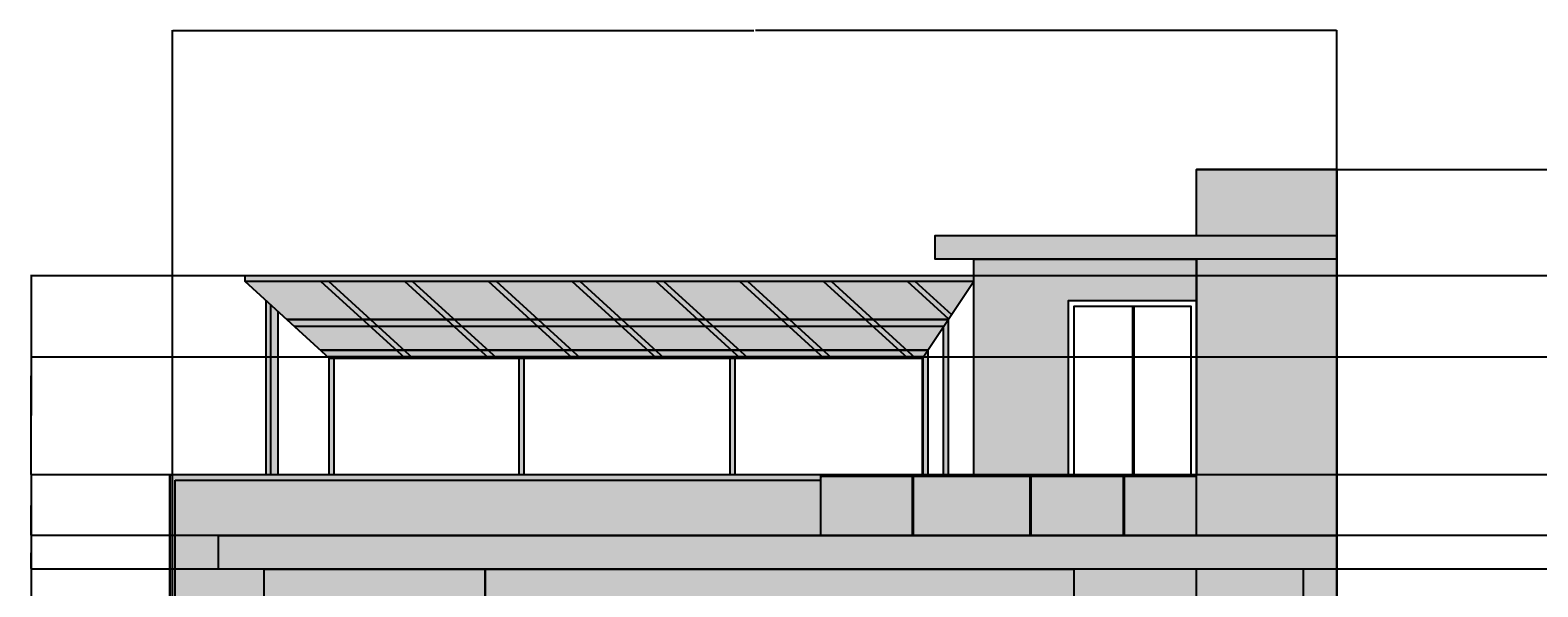
# Model space of a CAD drawing. Units: feet. Extents: x 2193 to 3502, y 890 to 1601.
# Tile 8 of 17: x 2193 to 2848, y 1360 to 1601. Entities that reach past the tile are written whole.
import ezdxf

# ---------------------------------------------------------------- set-up
doc = ezdxf.new("R2010")
doc.units = ezdxf.units.FT
for name, color, linetype, lineweight in [('A-ANNO-DIMS', 2, 'Continuous', 18), ('A-ELEV', 7, 'Continuous', 25), ('A-ELEV-PATT', 8, 'Continuous', 13)]:
    doc.layers.add(name, color=color, linetype=linetype, lineweight=lineweight)
doc.styles.get("Standard").update_dxf_attribs({"font": 'arial.ttf'})
doc.dimstyles.get("Standard").update_dxf_attribs({"dimtxt": 0.18, "dimasz": 0.18, "dimexe": 0.18, "dimexo": 0.0625, "dimgap": 0.09, "dimtad": 0, "dimtih": 1, "dimtoh": 1, "dimdec": 0, "dimzin": 0, "dimdsep": 46, "dimlunit": 3, "dimtxsty": 'Standard', "dimcen": 0.09, "dimadec": 0, "dimazin": 0, "dimtfac": 1, "dimtdec": 0, "dimtofl": 0, "dimtmove": 0, "dimatfit": 3, "dimfxl": 1, "dimtolj": 1, "dimtzin": 0, "dimarcsym": 0})

# ---------------------------------------------------------------- blocks, each defined once
blk = doc.blocks.new('*D20')
at = {"layer": 'A-ANNO-DIMS', "color": 0, "lineweight": -2, "transparency": 16777216}
for p, q in [((2933.15, 1408.48), (2193.56, 1408.48)), ((2193.74, 1408.3), (2193.74, 1240.94)), ((2193.74, 1073.21), (2193.74, 1240.57)), ((2934.31, 1073.03), (2193.56, 1073.03))]:
    blk.add_line(p, q, dxfattribs=at)
at = {"layer": 'A-ANNO-DIMS', "color": 0, "transparency": 16777216}
for points in [[(2193.71, 1408.3), (2193.77, 1408.3), (2193.74, 1408.48)], [(2193.71, 1073.21), (2193.77, 1073.21), (2193.74, 1073.03)]]:
    blk.add_solid(points, dxfattribs=at)
at = {"layer": 'Defpoints', "color": 0, "transparency": 16777216}
for p in [(2193.74, 1408.48), (2933.21, 1408.48), (2934.37, 1073.03)]:
    blk.add_point(p, dxfattribs=at)
at = {"layer": 'A-ANNO-DIMS', "color": 0, "transparency": 16777216, "insert": (2193.74, 1240.76), "char_height": 0.18, "attachment_point": 5}
blk.add_mtext('\\A1;335.45', dxfattribs=at)
blk = doc.blocks.new('*D21')
at = {"layer": 'A-ANNO-DIMS', "color": 0, "lineweight": -2, "transparency": 16777216}
for p, q in [((2965.66, 1494.8), (2193.56, 1494.8)), ((2193.74, 1494.62), (2193.74, 1451.82)), ((2193.74, 1408.66), (2193.74, 1451.46)), ((2974.89, 1408.48), (2193.56, 1408.48))]:
    blk.add_line(p, q, dxfattribs=at)
at = {"layer": 'A-ANNO-DIMS', "color": 0, "transparency": 16777216}
for points in [[(2193.71, 1494.62), (2193.77, 1494.62), (2193.74, 1494.8)], [(2193.71, 1408.66), (2193.77, 1408.66), (2193.74, 1408.48)]]:
    blk.add_solid(points, dxfattribs=at)
at = {"layer": 'Defpoints', "color": 0, "transparency": 16777216}
for p in [(2193.74, 1494.8), (2965.72, 1494.8), (2974.95, 1408.48)]:
    blk.add_point(p, dxfattribs=at)
at = {"layer": 'A-ANNO-DIMS', "color": 0, "transparency": 16777216, "insert": (2193.74, 1451.64), "char_height": 0.18, "attachment_point": 5}
blk.add_mtext('\\A1;86.32', dxfattribs=at)
blk = doc.blocks.new('*D26')
at = {"layer": 'A-ANNO-DIMS', "color": 0, "lineweight": -2, "transparency": 16777216}
for p, q in [((2255.16, 950.89), (2255.16, 1601.47)), ((2255.34, 1601.29), (2507.42, 1601.29)), ((2760.29, 1601.29), (2508.21, 1601.29)), ((2760.47, 1541.11), (2760.47, 1601.47))]:
    blk.add_line(p, q, dxfattribs=at)
at = {"layer": 'A-ANNO-DIMS', "color": 0, "transparency": 16777216}
for points in [[(2255.34, 1601.32), (2255.34, 1601.26), (2255.16, 1601.29)], [(2760.29, 1601.32), (2760.29, 1601.26), (2760.47, 1601.29)]]:
    blk.add_solid(points, dxfattribs=at)
at = {"layer": 'Defpoints', "color": 0, "transparency": 16777216}
for p in [(2760.47, 1601.29), (2760.47, 1541.04), (2255.16, 950.82)]:
    blk.add_point(p, dxfattribs=at)
at = {"layer": 'A-ANNO-DIMS', "color": 0, "transparency": 16777216, "insert": (2507.82, 1601.29), "char_height": 0.18, "attachment_point": 5}
blk.add_mtext('\\A1;505.3', dxfattribs=at)
blk = doc.blocks.new('*D31')
at = {"layer": 'A-ANNO-DIMS', "color": 0, "lineweight": -2, "transparency": 16777216}
for p, q in [((2760.54, 1541.04), (3501.85, 1541.04)), ((3501.67, 1540.86), (3501.67, 1246.12)), ((3501.67, 951), (3501.67, 1245.75)), ((2762.27, 950.82), (3501.85, 950.82))]:
    blk.add_line(p, q, dxfattribs=at)
at = {"layer": 'A-ANNO-DIMS', "color": 0, "transparency": 16777216}
for points in [[(3501.64, 1540.86), (3501.7, 1540.86), (3501.67, 1541.04)], [(3501.64, 951), (3501.7, 951), (3501.67, 950.82)]]:
    blk.add_solid(points, dxfattribs=at)
at = {"layer": 'Defpoints', "color": 0, "transparency": 16777216}
for p in [(2760.47, 1541.04), (3501.67, 1541.04), (2762.2, 950.82)]:
    blk.add_point(p, dxfattribs=at)
at = {"layer": 'A-ANNO-DIMS', "color": 0, "transparency": 16777216, "insert": (3501.67, 1245.93), "char_height": 0.18, "attachment_point": 5}
blk.add_mtext('\\A1;590.2', dxfattribs=at)
blk = doc.blocks.new('*D33')
at = {"layer": 'A-ANNO-DIMS', "color": 0, "lineweight": -2, "transparency": 16777216}
for p, q in [((2253.93, 1408.48), (2193.56, 1408.48)), ((2193.74, 1408.3), (2193.74, 1240.94)), ((2193.74, 1073.21), (2193.74, 1240.57)), ((2255.09, 1073.03), (2193.56, 1073.03))]:
    blk.add_line(p, q, dxfattribs=at)
at = {"layer": 'A-ANNO-DIMS', "color": 0, "transparency": 16777216}
for points in [[(2193.71, 1408.3), (2193.77, 1408.3), (2193.74, 1408.48)], [(2193.71, 1073.21), (2193.77, 1073.21), (2193.74, 1073.03)]]:
    blk.add_solid(points, dxfattribs=at)
at = {"layer": 'Defpoints', "color": 0, "transparency": 16777216}
for p in [(2193.74, 1408.48), (2253.99, 1408.48), (2255.16, 1073.03)]:
    blk.add_point(p, dxfattribs=at)
at = {"layer": 'A-ANNO-DIMS', "color": 0, "transparency": 16777216, "insert": (2193.74, 1240.76), "char_height": 0.18, "attachment_point": 5}
blk.add_mtext('\\A1;335.45', dxfattribs=at)
blk = doc.blocks.new('*D34')
at = {"layer": 'A-ANNO-DIMS', "color": 0, "lineweight": -2, "transparency": 16777216}
for p, q in [((2286.44, 1494.8), (2193.56, 1494.8)), ((2193.74, 1494.62), (2193.74, 1451.82)), ((2193.74, 1408.66), (2193.74, 1451.46)), ((2295.67, 1408.48), (2193.56, 1408.48))]:
    blk.add_line(p, q, dxfattribs=at)
at = {"layer": 'A-ANNO-DIMS', "color": 0, "transparency": 16777216}
for points in [[(2193.71, 1494.62), (2193.77, 1494.62), (2193.74, 1494.8)], [(2193.71, 1408.66), (2193.77, 1408.66), (2193.74, 1408.48)]]:
    blk.add_solid(points, dxfattribs=at)
at = {"layer": 'Defpoints', "color": 0, "transparency": 16777216}
for p in [(2193.74, 1494.8), (2286.5, 1494.8), (2295.74, 1408.48)]:
    blk.add_point(p, dxfattribs=at)
at = {"layer": 'A-ANNO-DIMS', "color": 0, "transparency": 16777216, "insert": (2193.74, 1451.64), "char_height": 0.18, "attachment_point": 5}
blk.add_mtext('\\A1;86.32', dxfattribs=at)
blk = doc.blocks.new('*D37')
at = {"layer": 'A-ANNO-DIMS', "color": 0, "lineweight": -2, "transparency": 16777216}
for p, q in [((2974.05, 1367.57), (2193.56, 1367.57)), ((2193.74, 1367.39), (2193.74, 1318.3)), ((2193.74, 1268.84), (2193.74, 1317.93)), ((2974.05, 1268.66), (2193.56, 1268.66))]:
    blk.add_line(p, q, dxfattribs=at)
at = {"layer": 'A-ANNO-DIMS', "color": 0, "transparency": 16777216}
for points in [[(2193.71, 1367.39), (2193.77, 1367.39), (2193.74, 1367.57)], [(2193.71, 1268.84), (2193.77, 1268.84), (2193.74, 1268.66)]]:
    blk.add_solid(points, dxfattribs=at)
at = {"layer": 'Defpoints', "color": 0, "transparency": 16777216}
for p in [(2193.74, 1367.57), (2974.12, 1367.57), (2974.12, 1268.66)]:
    blk.add_point(p, dxfattribs=at)
at = {"layer": 'A-ANNO-DIMS', "color": 0, "transparency": 16777216, "insert": (2193.74, 1318.12), "char_height": 0.18, "attachment_point": 5}
blk.add_mtext('\\A1;98.91', dxfattribs=at)
blk = doc.blocks.new('*D38')
at = {"layer": 'A-ANNO-DIMS', "color": 0, "lineweight": -2, "transparency": 16777216}
for p, q in [((2954.2, 1382.08), (2193.56, 1382.08)), ((2193.74, 1381.9), (2193.74, 1375.01)), ((2193.74, 1367.75), (2193.74, 1374.64)), ((2954.2, 1367.57), (2193.56, 1367.57))]:
    blk.add_line(p, q, dxfattribs=at)
at = {"layer": 'A-ANNO-DIMS', "color": 0, "transparency": 16777216}
for points in [[(2193.71, 1381.9), (2193.77, 1381.9), (2193.74, 1382.08)], [(2193.71, 1367.75), (2193.77, 1367.75), (2193.74, 1367.57)]]:
    blk.add_solid(points, dxfattribs=at)
at = {"layer": 'Defpoints', "color": 0, "transparency": 16777216}
for p in [(2193.74, 1382.08), (2954.26, 1382.08), (2954.26, 1367.57)]:
    blk.add_point(p, dxfattribs=at)
at = {"layer": 'A-ANNO-DIMS', "color": 0, "transparency": 16777216, "insert": (2193.74, 1374.83), "char_height": 0.18, "attachment_point": 5}
blk.add_mtext('\\A1;14.502', dxfattribs=at)
blk = doc.blocks.new('*D39')
at = {"layer": 'A-ANNO-DIMS', "color": 0, "lineweight": -2, "transparency": 16777216}
for p, q in [((2933.15, 1408.48), (2193.56, 1408.48)), ((2193.74, 1408.3), (2193.74, 1395.46)), ((2193.74, 1382.26), (2193.74, 1395.1)), ((2954.2, 1382.08), (2193.56, 1382.08))]:
    blk.add_line(p, q, dxfattribs=at)
at = {"layer": 'A-ANNO-DIMS', "color": 0, "transparency": 16777216}
for points in [[(2193.71, 1408.3), (2193.77, 1408.3), (2193.74, 1408.48)], [(2193.71, 1382.26), (2193.77, 1382.26), (2193.74, 1382.08)]]:
    blk.add_solid(points, dxfattribs=at)
at = {"layer": 'Defpoints', "color": 0, "transparency": 16777216}
for p in [(2193.74, 1408.48), (2933.21, 1408.48), (2954.26, 1382.08)]:
    blk.add_point(p, dxfattribs=at)
at = {"layer": 'A-ANNO-DIMS', "color": 0, "transparency": 16777216, "insert": (2193.74, 1395.28), "char_height": 0.18, "attachment_point": 5}
blk.add_mtext('\\A1;26.405', dxfattribs=at)
blk = doc.blocks.new('*D58')
at = {"layer": 'A-ANNO-DIMS', "color": 0, "lineweight": -2, "transparency": 16777216}
for p, q in [((3001.83, 1459.6), (2193.56, 1459.6)), ((2193.74, 1459.42), (2193.74, 1434.22)), ((2193.74, 1408.66), (2193.74, 1433.86)), ((2974.89, 1408.48), (2193.56, 1408.48))]:
    blk.add_line(p, q, dxfattribs=at)
at = {"layer": 'A-ANNO-DIMS', "color": 0, "transparency": 16777216}
for points in [[(2193.71, 1459.42), (2193.77, 1459.42), (2193.74, 1459.6)], [(2193.71, 1408.66), (2193.77, 1408.66), (2193.74, 1408.48)]]:
    blk.add_solid(points, dxfattribs=at)
at = {"layer": 'Defpoints', "color": 0, "transparency": 16777216}
for p in [(2193.74, 1459.6), (3001.89, 1459.6), (2974.95, 1408.48)]:
    blk.add_point(p, dxfattribs=at)
at = {"layer": 'A-ANNO-DIMS', "color": 0, "transparency": 16777216, "insert": (2193.74, 1434.04), "char_height": 0.18, "attachment_point": 5}
blk.add_mtext('\\A1;51.12', dxfattribs=at)

msp = doc.modelspace()

# ---------------------------------------------------------------- hatches: boundary and pattern name
at = {"layer": 'A-ELEV-PATT'}
h = msp.add_hatch(color=256, dxfattribs=at)
h.dxf.hatch_style = 1
h.paths.add_polyline_path([(2760.4733, 1541.0441), (2699.6322, 1541.0441), (2699.6322, 1512.3957), (2760.4733, 1512.3957)])
h.paths.add_polyline_path([(2760.4733, 1502.0763), (2699.6322, 1502.0763), (2699.6322, 1382.0763), (2760.4733, 1382.0763)])
h.paths.add_polyline_path([(2745.971, 1367.5739), (2699.6322, 1367.5739), (2699.6322, 1089.3627), (2760.4733, 1089.3627), (2760.4733, 1166.2327), (2745.971, 1166.2327)])
h.paths.add_polyline_path([(2754.7661, 1011.1246), (2690.9216, 1011.1246), (2690.9216, 993.3923), (2754.7661, 993.3923)])
h.paths.add_polyline_path([(2689.6008, 1011.1246), (2625.7563, 1011.1246), (2625.7563, 993.3923), (2689.6008, 993.3923)])
h.paths.add_polyline_path([(2599.6883, 1249.8256), (2598.591, 1249.8256), (2598.591, 1233.561), (2599.6883, 1233.561)])
h.paths.add_polyline_path([(2602.5204, 1247.0422), (2601.423, 1247.0422), (2601.423, 1233.561), (2602.5204, 1233.561)])
h.paths.add_polyline_path([(2606.5316, 1250.4403), (2605.4342, 1250.4403), (2605.4342, 1233.561), (2606.5316, 1233.561)])
h.paths.add_polyline_path([(2609.5836, 1248.4363), (2608.4862, 1248.4363), (2608.4862, 1233.561), (2609.5836, 1233.561)])
h.paths.add_polyline_path([(2613.8564, 1243.2956), (2612.759, 1243.2956), (2612.759, 1233.561), (2613.8564, 1233.561)])
h.paths.add_polyline_path([(2616.5596, 1249.6561), (2615.4622, 1249.6561), (2615.4622, 1233.561), (2616.5596, 1233.561)])
h.paths.add_polyline_path([(2599.6883, 1233.561), (2598.591, 1233.561), (2598.591, 1224.865), (2599.6883, 1224.865)])
h.paths.add_polyline_path([(2602.5204, 1233.561), (2601.423, 1233.561), (2601.423, 1224.865), (2602.5204, 1224.865)])
h.paths.add_polyline_path([(2606.5316, 1233.561), (2605.4342, 1233.561), (2605.4342, 1224.865), (2606.5316, 1224.865)])
h.paths.add_polyline_path([(2609.5836, 1233.561), (2608.4862, 1233.561), (2608.4862, 1224.865), (2609.5836, 1224.865)])
h.paths.add_polyline_path([(2613.8564, 1233.561), (2612.759, 1233.561), (2612.759, 1224.865), (2613.8564, 1224.865)])
h.paths.add_polyline_path([(2616.5596, 1233.561), (2615.4622, 1233.561), (2615.4622, 1224.865), (2616.5596, 1224.865)])
h.paths.add_polyline_path([(2599.6883, 1224.865), (2598.591, 1224.865), (2598.591, 1115.2331), (2599.6883, 1115.2331)])
h.paths.add_polyline_path([(2602.5204, 1224.865), (2601.423, 1224.865), (2601.423, 1112.4498), (2602.5204, 1112.4498)])
h.paths.add_polyline_path([(2606.5316, 1224.865), (2605.4342, 1224.865), (2605.4342, 1115.8479), (2606.5316, 1115.8479)])
h.paths.add_polyline_path([(2609.5836, 1224.865), (2608.4862, 1224.865), (2608.4862, 1113.8439), (2609.5836, 1113.8439)])
h.paths.add_polyline_path([(2616.5596, 1224.865), (2615.4622, 1224.865), (2615.4622, 1115.0637), (2616.5596, 1115.0637)])
h.paths.add_polyline_path([(2613.8564, 1224.865), (2612.759, 1224.865), (2612.759, 1108.7032), (2613.8564, 1108.7032)])
h = msp.add_hatch(color=256, dxfattribs=at)
h.dxf.hatch_style = 1
h.paths.add_polyline_path([(2760.4733, 1512.3957), (2586.1736, 1512.3957), (2586.1736, 1502.0763), (2602.8648, 1502.0763), (2699.5726, 1502.0763), (2699.6322, 1502.0763), (2760.4733, 1502.0763)])
h.paths.add_polyline_path([(2760.4733, 1382.0763), (2275.0482, 1382.0763), (2275.0482, 1367.5739), (2745.971, 1367.5739), (2745.971, 1166.2327), (2760.4733, 1166.2327)])
h.paths.add_polyline_path([(2468.2854, 1266.7092), (2294.8992, 1266.7092), (2294.8992, 1079.031), (2468.2854, 1079.031)])
h.paths.add_polyline_path([(2301.4984, 1260.11), (2461.6863, 1260.11), (2461.6863, 1085.6301), (2301.4984, 1085.6301)], flags=16)
h.paths.add_polyline_path([(2452.7821, 1241.1967), (2452.7821, 1217.2819), (2454.6216, 1217.2819), (2454.6216, 1133.1367), (2461.6863, 1133.1367), (2461.6863, 1132.3937), (2381.7172, 1132.3937), (2381.7172, 1085.6301), (2381.4675, 1085.6301), (2381.4675, 1132.3937), (2301.4984, 1132.3937), (2301.4984, 1133.1367), (2301.4984, 1217.2819), (2390.8933, 1217.2819), (2390.8933, 1241.1967)], flags=0)
h.paths.add_polyline_path([(2372.4936, 1214.8367), (2372.4936, 1133.1367), (2371.1246, 1133.1367), (2371.1246, 1214.8367), (2337.2323, 1214.8367), (2337.2323, 1133.1367), (2335.8632, 1133.1367), (2335.8632, 1214.8367), (2337.2323, 1214.8367)], flags=0)
h = msp.add_hatch(color=256, dxfattribs=at)
h.dxf.hatch_style = 1
h.paths.add_polyline_path([(2390.8933, 1367.5739), (2294.8992, 1367.5739), (2294.8992, 1329.5765), (2390.8933, 1329.5765)])
h.paths.add_polyline_path([(2489.6169, 1055.3069), (2585.8844, 1055.3069), (2585.8844, 1032.1935), (2620.0491, 1032.1935), (2620.0491, 1073.031), (2452.7821, 1073.031), (2452.7821, 1032.1935), (2489.6169, 1032.1935)])
h.paths.add_polyline_path([(2754.7661, 1073.031), (2654.2841, 1073.031), (2654.2841, 1047.0961), (2754.7661, 1047.0961)])
h.paths.add_polyline_path([(2643.9681, 1484.1152), (2699.5726, 1484.1152), (2699.5726, 1502.0763), (2602.8648, 1502.0763), (2602.8648, 1408.4814), (2643.9681, 1408.4814)])
h.paths.add_polyline_path([(2699.6322, 1367.5739), (2646.2844, 1367.5739), (2646.2844, 1268.6599), (2647.1841, 1268.6599), (2647.1841, 1329.5765), (2699.6322, 1329.5765)])
h.paths.add_polyline_path([(2699.6322, 1224.865), (2616.5596, 1224.865), (2616.5596, 1133.8558), (2647.1841, 1133.8558), (2647.1841, 1194.7724), (2699.6322, 1194.7724)])
h = msp.add_hatch(color=256, dxfattribs=at)
h.dxf.hatch_style = 1
h.paths.add_polyline_path([(2760.4733, 956.8829), (2754.7661, 956.8829), (2625.7563, 956.8829), (2626.1971, 953.031), (2626.1971, 950.8228), (2762.2048, 950.8228)])
h.paths.add_polyline_path([(2587.7084, 958.9555), (2461.0056, 958.9555), (2461.0056, 953.031), (2587.7084, 953.031)])
h.paths.add_polyline_path([(2480.0809, 960.0129), (2463.2716, 960.0129), (2461.0056, 958.9555), (2480.0809, 958.9555)])
h.paths.add_polyline_path([(2514.917, 960.0129), (2500.4779, 960.0129), (2500.4779, 958.9555), (2514.917, 958.9555)])
h.paths.add_polyline_path([(2552.6959, 960.0129), (2538.2568, 960.0129), (2538.2568, 958.9555), (2552.6959, 958.9555)])
h.paths.add_polyline_path([(2588.4279, 960.0129), (2573.0929, 960.0129), (2573.0929, 958.9555), (2587.7084, 958.9555)])
h.paths.add_polyline_path([(2588.4279, 960.0129), (2587.7084, 958.9555), (2587.7084, 953.031), (2588.4279, 953.031)])
h.paths.add_polyline_path([(2461.0056, 956.8829), (2261.443, 956.8829), (2255.1574, 953.031), (2461.0056, 953.031)])
h.paths.add_polyline_path([(2625.7563, 956.8829), (2600.3918, 956.8829), (2600.3918, 953.031), (2626.1971, 953.031)])
h.paths.add_polyline_path([(2600.3918, 956.8829), (2588.4279, 956.8829), (2588.4279, 953.031), (2600.3918, 953.031)])
h.paths.add_polyline_path([(2602.8648, 1494.8043), (2286.5029, 1494.8043), (2286.5029, 1492.5146), (2602.8648, 1492.5146)])
h.paths.add_polyline_path([(2322.8578, 1492.5146), (2319.4392, 1492.5146), (2337.7496, 1475.8561), (2341.1681, 1475.8561)])
h.paths.add_polyline_path([(2341.1681, 1475.8561), (2337.7496, 1475.8561), (2341.051, 1472.8525), (2344.4696, 1472.8525)])
h.paths.add_polyline_path([(2344.4696, 1472.8525), (2341.051, 1472.8525), (2352.3124, 1462.6071), (2355.731, 1462.6071)])
h.paths.add_polyline_path([(2355.731, 1462.6071), (2352.3124, 1462.6071), (2355.6139, 1459.6035), (2359.0325, 1459.6035)])
h.paths.add_polyline_path([(2325.1721, 1459.1592), (2323.1659, 1459.1592), (2323.1659, 1408.4814), (2325.1721, 1408.4814)])
h.paths.add_polyline_path([(2297.6937, 1482.3334), (2295.7368, 1484.1138), (2295.7368, 1408.4814), (2297.6937, 1408.4814)])
h.paths.add_polyline_path([(2300.8766, 1479.4377), (2297.6937, 1482.3334), (2297.6937, 1408.4814), (2300.8766, 1408.4814)])
h.paths.add_polyline_path([(2337.7496, 1475.8561), (2304.8133, 1475.8561), (2308.1148, 1472.8525), (2341.051, 1472.8525)])
h.paths.add_polyline_path([(2352.3124, 1462.6071), (2319.3762, 1462.6071), (2322.6776, 1459.6035), (2355.6139, 1459.6035)])
h.paths.add_polyline_path([(2374.1044, 1475.8561), (2341.1681, 1475.8561), (2344.4696, 1472.8525), (2377.4059, 1472.8525)])
h.paths.add_polyline_path([(2388.6672, 1462.6071), (2355.731, 1462.6071), (2359.0325, 1459.6035), (2391.9687, 1459.6035)])
h.paths.add_polyline_path([(2392.0858, 1462.6071), (2388.6672, 1462.6071), (2391.9687, 1459.6035), (2395.3873, 1459.6035)])
h.paths.add_polyline_path([(2380.8245, 1472.8525), (2377.4059, 1472.8525), (2388.6672, 1462.6071), (2392.0858, 1462.6071)])
h.paths.add_polyline_path([(2377.523, 1475.8561), (2374.1044, 1475.8561), (2377.4059, 1472.8525), (2380.8245, 1472.8525)])
h.paths.add_polyline_path([(2359.2126, 1492.5146), (2355.794, 1492.5146), (2374.1044, 1475.8561), (2377.523, 1475.8561)])
h.paths.add_polyline_path([(2395.5674, 1492.5146), (2392.1488, 1492.5146), (2410.4592, 1475.8561), (2413.8778, 1475.8561)])
h.paths.add_polyline_path([(2410.4592, 1475.8561), (2377.523, 1475.8561), (2380.8245, 1472.8525), (2413.7607, 1472.8525)])
h.paths.add_polyline_path([(2413.8778, 1475.8561), (2410.4592, 1475.8561), (2413.7607, 1472.8525), (2417.1793, 1472.8525)])
h.paths.add_polyline_path([(2417.1793, 1472.8525), (2413.7607, 1472.8525), (2425.022, 1462.6071), (2428.4406, 1462.6071)])
h.paths.add_polyline_path([(2425.022, 1462.6071), (2392.0858, 1462.6071), (2395.3873, 1459.6035), (2428.3235, 1459.6035)])
h.paths.add_polyline_path([(2428.4406, 1462.6071), (2425.022, 1462.6071), (2428.3235, 1459.6035), (2431.7421, 1459.6035)])
h.paths.add_polyline_path([(2461.3769, 1462.6071), (2428.4406, 1462.6071), (2431.7421, 1459.6035), (2464.6784, 1459.6035)])
h.paths.add_polyline_path([(2577.3415, 1492.5146), (2573.9229, 1492.5146), (2591.9256, 1476.1361), (2593.2177, 1478.0707)])
h.paths.add_polyline_path([(2540.9867, 1492.5146), (2537.5681, 1492.5146), (2555.8785, 1475.8561), (2559.2971, 1475.8561)])
h.paths.add_polyline_path([(2591.7386, 1475.8561), (2559.2971, 1475.8561), (2562.5986, 1472.8525), (2589.7325, 1472.8525)])
h.paths.add_polyline_path([(2555.8785, 1475.8561), (2522.9423, 1475.8561), (2526.2437, 1472.8525), (2559.18, 1472.8525)])
h.paths.add_polyline_path([(2559.2971, 1475.8561), (2555.8785, 1475.8561), (2559.18, 1472.8525), (2562.5986, 1472.8525)])
h.paths.add_polyline_path([(2562.5986, 1472.8525), (2559.18, 1472.8525), (2570.4413, 1462.6071), (2573.8599, 1462.6071)])
h.paths.add_polyline_path([(2570.4413, 1462.6071), (2537.5051, 1462.6071), (2540.8066, 1459.6035), (2573.7428, 1459.6035)])
h.paths.add_polyline_path([(2582.8896, 1462.6071), (2573.8599, 1462.6071), (2577.1614, 1459.6035), (2580.8835, 1459.6035)])
h.paths.add_polyline_path([(2573.8599, 1462.6071), (2570.4413, 1462.6071), (2573.7428, 1459.6035), (2577.1614, 1459.6035)])
h.paths.add_polyline_path([(2591.7386, 1475.8561), (2589.7325, 1472.8525), (2589.7325, 1408.4814), (2591.7386, 1408.4814)])
h.paths.add_polyline_path([(2582.8896, 1462.6071), (2580.8835, 1459.6035), (2580.8835, 1408.4814), (2582.8896, 1408.4814)])
h.paths.add_polyline_path([(2504.6319, 1492.5146), (2501.2133, 1492.5146), (2519.5237, 1475.8561), (2522.9423, 1475.8561)])
h.paths.add_polyline_path([(2534.0865, 1462.6071), (2501.1503, 1462.6071), (2504.4518, 1459.6035), (2537.388, 1459.6035)])
h.paths.add_polyline_path([(2537.5051, 1462.6071), (2534.0865, 1462.6071), (2537.388, 1459.6035), (2540.8066, 1459.6035)])
h.paths.add_polyline_path([(2526.2437, 1472.8525), (2522.8252, 1472.8525), (2534.0865, 1462.6071), (2537.5051, 1462.6071)])
h.paths.add_polyline_path([(2522.9423, 1475.8561), (2519.5237, 1475.8561), (2522.8252, 1472.8525), (2526.2437, 1472.8525)])
h.paths.add_polyline_path([(2519.5237, 1475.8561), (2486.5874, 1475.8561), (2489.8889, 1472.8525), (2522.8252, 1472.8525)])
h.paths.add_polyline_path([(2483.1689, 1475.8561), (2450.2326, 1475.8561), (2453.5341, 1472.8525), (2486.4703, 1472.8525)])
h.paths.add_polyline_path([(2486.5874, 1475.8561), (2483.1689, 1475.8561), (2486.4703, 1472.8525), (2489.8889, 1472.8525)])
h.paths.add_polyline_path([(2468.277, 1492.5146), (2464.8585, 1492.5146), (2483.1689, 1475.8561), (2486.5874, 1475.8561)])
h.paths.add_polyline_path([(2489.8889, 1472.8525), (2486.4703, 1472.8525), (2497.7317, 1462.6071), (2501.1503, 1462.6071)])
h.paths.add_polyline_path([(2497.7317, 1462.6071), (2464.7955, 1462.6071), (2468.0969, 1459.6035), (2501.0332, 1459.6035)])
h.paths.add_polyline_path([(2501.1503, 1462.6071), (2497.7317, 1462.6071), (2501.0332, 1459.6035), (2504.4518, 1459.6035)])
h.paths.add_polyline_path([(2464.7955, 1462.6071), (2461.3769, 1462.6071), (2464.6784, 1459.6035), (2468.0969, 1459.6035)])
h.paths.add_polyline_path([(2453.5341, 1472.8525), (2450.1155, 1472.8525), (2461.3769, 1462.6071), (2464.7955, 1462.6071)])
h.paths.add_polyline_path([(2431.9222, 1492.5146), (2428.5036, 1492.5146), (2446.814, 1475.8561), (2450.2326, 1475.8561)])
h.paths.add_polyline_path([(2446.814, 1475.8561), (2413.8778, 1475.8561), (2417.1793, 1472.8525), (2450.1155, 1472.8525)])
h.paths.add_polyline_path([(2450.2326, 1475.8561), (2446.814, 1475.8561), (2450.1155, 1472.8525), (2453.5341, 1472.8525)])
h.paths.add_polyline_path([(2407.5925, 1459.1592), (2405.5863, 1459.1592), (2405.5863, 1408.4814), (2407.5925, 1408.4814)])
h.paths.add_polyline_path([(2499.2252, 1459.1592), (2497.2191, 1459.1592), (2497.2191, 1408.4814), (2499.2252, 1408.4814)])
h = msp.add_hatch(color=256, dxfattribs=at)
h.dxf.hatch_style = 1
h.paths.add_polyline_path([(2319.4392, 1492.5146), (2286.5029, 1492.5146), (2304.8133, 1475.8561), (2337.7496, 1475.8561)])
h.paths.add_polyline_path([(2355.794, 1492.5146), (2322.8578, 1492.5146), (2341.1681, 1475.8561), (2374.1044, 1475.8561)])
h.paths.add_polyline_path([(2392.1488, 1492.5146), (2359.2126, 1492.5146), (2377.523, 1475.8561), (2410.4592, 1475.8561)])
h.paths.add_polyline_path([(2377.4059, 1472.8525), (2344.4696, 1472.8525), (2355.731, 1462.6071), (2388.6672, 1462.6071)])
h.paths.add_polyline_path([(2413.7607, 1472.8525), (2380.8245, 1472.8525), (2392.0858, 1462.6071), (2425.022, 1462.6071)])
h.paths.add_polyline_path([(2341.051, 1472.8525), (2308.1148, 1472.8525), (2319.3762, 1462.6071), (2352.3124, 1462.6071)])
h.paths.add_polyline_path([(2428.5036, 1492.5146), (2395.5674, 1492.5146), (2413.8778, 1475.8561), (2446.814, 1475.8561)])
h.paths.add_polyline_path([(2464.8585, 1492.5146), (2431.9222, 1492.5146), (2450.2326, 1475.8561), (2483.1689, 1475.8561)])
h.paths.add_polyline_path([(2450.1155, 1472.8525), (2417.1793, 1472.8525), (2428.4406, 1462.6071), (2461.3769, 1462.6071)])
h.paths.add_polyline_path([(2486.4703, 1472.8525), (2453.5341, 1472.8525), (2464.7955, 1462.6071), (2497.7317, 1462.6071)])
h.paths.add_polyline_path([(2602.8648, 1492.5146), (2577.3415, 1492.5146), (2593.2177, 1478.0707)])
h.paths.add_polyline_path([(2573.9229, 1492.5146), (2540.9867, 1492.5146), (2559.2971, 1475.8561), (2591.7386, 1475.8561), (2591.9256, 1476.1361)])
h.paths.add_polyline_path([(2589.7325, 1472.8525), (2562.5986, 1472.8525), (2573.8599, 1462.6071), (2582.8896, 1462.6071)])
h.paths.add_polyline_path([(2559.18, 1472.8525), (2526.2437, 1472.8525), (2537.5051, 1462.6071), (2570.4413, 1462.6071)])
h.paths.add_polyline_path([(2537.5681, 1492.5146), (2504.6319, 1492.5146), (2522.9423, 1475.8561), (2555.8785, 1475.8561)])
h.paths.add_polyline_path([(2501.2133, 1492.5146), (2468.277, 1492.5146), (2486.5874, 1475.8561), (2519.5237, 1475.8561)])
h.paths.add_polyline_path([(2522.8252, 1472.8525), (2489.8889, 1472.8525), (2501.1503, 1462.6071), (2534.0865, 1462.6071)])
h = msp.add_hatch(color=256, dxfattribs=at)
h.dxf.hatch_style = 1
h.paths.add_polyline_path([(2256.3232, 1406.15), (2536.5416, 1406.15), (2536.5416, 1408.4814), (2253.9917, 1408.4814), (2253.9917, 1089.3627), (2255.1574, 1089.3627), (2256.3232, 1089.3627)])
h = msp.add_hatch(color=256, dxfattribs=at)
h.dxf.hatch_style = 1
h.paths.add_polyline_path([(2576.3428, 1407.7384), (2536.5416, 1407.7384), (2536.5416, 1406.15), (2536.5416, 1382.0763), (2576.3428, 1382.0763)])
h.paths.add_polyline_path([(2627.3548, 1407.7384), (2576.5924, 1407.7384), (2576.5924, 1382.0763), (2627.3548, 1382.0763)])
h.paths.add_polyline_path([(2667.9236, 1407.7384), (2627.6045, 1407.7384), (2627.6045, 1382.0763), (2667.9236, 1382.0763)])
h.paths.add_polyline_path([(2699.6322, 1407.7384), (2668.1733, 1407.7384), (2668.1733, 1382.0763), (2699.6322, 1382.0763)])
h.paths.add_polyline_path([(2497.5717, 1323.2248), (2470.7305, 1323.2248), (2470.7305, 1271.105), (2497.5717, 1271.105)])
h.paths.add_polyline_path([(2577.3219, 1323.2248), (2500.599, 1323.2248), (2500.599, 1271.105), (2577.3219, 1271.105)])
h.paths.add_polyline_path([(2388.4482, 1327.1314), (2343.4244, 1327.1314), (2343.4244, 1268.6599), (2388.4482, 1268.6599)])
h.paths.add_polyline_path([(2342.3682, 1327.1314), (2297.3443, 1327.1314), (2297.3443, 1268.6599), (2342.3682, 1268.6599)])
h.paths.add_polyline_path([(2335.8632, 1214.8367), (2301.4984, 1214.8367), (2301.4984, 1133.1367), (2335.8632, 1133.1367)])
h.paths.add_polyline_path([(2371.1246, 1214.8367), (2337.2323, 1214.8367), (2337.2323, 1133.1367), (2371.1246, 1133.1367)])
h.paths.add_polyline_path([(2390.8933, 1214.8367), (2372.4936, 1214.8367), (2372.4936, 1133.1367), (2390.8933, 1133.1367)])
h.paths.add_polyline_path([(2577.3219, 1188.4208), (2500.599, 1188.4208), (2500.599, 1136.3009), (2577.3219, 1136.3009)])
h.paths.add_polyline_path([(2497.5717, 1188.4208), (2470.7305, 1188.4208), (2470.7305, 1136.3009), (2497.5717, 1136.3009)])
h.paths.add_polyline_path([(2381.4675, 1132.3937), (2301.4984, 1132.3937), (2301.4984, 1085.6301), (2381.4675, 1085.6301)])
h.paths.add_polyline_path([(2461.6863, 1132.3937), (2381.7172, 1132.3937), (2381.7172, 1085.6301), (2461.6863, 1085.6301)])
h.paths.add_polyline_path([(2494.0463, 1133.1128), (2468.2854, 1133.1128), (2468.2854, 1089.3627), (2494.0463, 1089.3627)])
h.paths.add_polyline_path([(2517.7591, 1133.1128), (2494.296, 1133.1128), (2494.296, 1089.3627), (2517.7591, 1089.3627)])
h.paths.add_polyline_path([(2667.9236, 1133.1128), (2636.5184, 1133.1128), (2636.5184, 1089.3627), (2667.9236, 1089.3627)])
h.paths.add_polyline_path([(2699.6322, 1133.1128), (2668.1733, 1133.1128), (2668.1733, 1089.3627), (2699.6322, 1089.3627)])
h.paths.add_polyline_path([(2651.839, 1070.5859), (2638.7977, 1070.5859), (2638.7977, 1047.0961), (2651.839, 1047.0961)])
h.paths.add_polyline_path([(2637.6317, 1070.5859), (2625.7563, 1070.5859), (2625.7563, 1047.0961), (2637.6317, 1047.0961)])
h.paths.add_polyline_path([(2583.4393, 1052.8618), (2515.9216, 1052.8618), (2515.9216, 1032.1935), (2583.4393, 1032.1935)])
h.paths.add_polyline_path([(2514.4293, 1052.8618), (2492.062, 1052.8618), (2492.062, 1032.1935), (2514.4293, 1032.1935)])
h.paths.add_polyline_path([(2388.4482, 1038.8658), (2348.7682, 1038.8658), (2348.7682, 988.9597), (2388.4482, 988.9597)])
h.paths.add_polyline_path([(2346.3231, 1038.8658), (2309.0883, 1038.8658), (2309.0883, 988.9597), (2346.3231, 988.9597)])
h.paths.add_polyline_path([(2667.9236, 1267.9169), (2636.5184, 1267.9169), (2636.5184, 1241.1967), (2667.9236, 1241.1967)])
h.paths.add_polyline_path([(2699.6322, 1267.9169), (2668.1733, 1267.9169), (2668.1733, 1241.1967), (2699.6322, 1241.1967)])
h.paths.add_polyline_path([(2517.7591, 1267.9169), (2494.296, 1267.9169), (2494.296, 1241.1967), (2517.7591, 1241.1967)])
h.paths.add_polyline_path([(2494.0463, 1267.9169), (2468.2854, 1267.9169), (2468.2854, 1266.7092), (2468.2854, 1241.1967), (2494.0463, 1241.1967)])
h = msp.add_hatch(color=256, dxfattribs=at)
h.dxf.hatch_style = 1
h.paths.add_polyline_path([(2294.8992, 1367.5739), (2275.0482, 1367.5739), (2275.0482, 1382.0763), (2536.5416, 1382.0763), (2536.5416, 1406.15), (2256.3232, 1406.15), (2256.3232, 1089.3627), (2255.1574, 1089.3627), (2255.1574, 1073.031), (2294.8992, 1073.031)])
h.paths.add_polyline_path([(2517.7591, 1241.1967), (2468.2854, 1241.1967), (2468.2854, 1224.865), (2598.591, 1224.865), (2598.591, 1233.561), (2517.7591, 1233.561)])
h.paths.add_polyline_path([(2699.6322, 1241.1967), (2636.5184, 1241.1967), (2636.5184, 1233.561), (2616.5596, 1233.561), (2616.5596, 1224.865), (2699.6322, 1224.865)])
h.paths.add_polyline_path([(2615.4622, 1233.561), (2613.8564, 1233.561), (2613.8564, 1224.865), (2615.4622, 1224.865)])
h.paths.add_polyline_path([(2612.759, 1233.561), (2609.5836, 1233.561), (2609.5836, 1224.865), (2612.759, 1224.865)])
h.paths.add_polyline_path([(2608.4862, 1233.561), (2606.5316, 1233.561), (2606.5316, 1224.865), (2608.4862, 1224.865)])
h.paths.add_polyline_path([(2605.4342, 1233.561), (2602.5204, 1233.561), (2602.5204, 1224.865), (2605.4342, 1224.865)])
h.paths.add_polyline_path([(2601.423, 1233.561), (2599.6883, 1233.561), (2599.6883, 1224.865), (2601.423, 1224.865)])
h.paths.add_polyline_path([(2517.7591, 1089.3627), (2468.2854, 1089.3627), (2468.2854, 1079.031), (2294.8992, 1079.031), (2294.8992, 1073.031), (2390.8933, 1073.031), (2452.7821, 1073.031), (2760.4733, 1073.031), (2760.4733, 1089.3627), (2699.6322, 1089.3627), (2636.5184, 1089.3627), (2636.5184, 1081.7269), (2517.7591, 1081.7269)])
h = msp.add_hatch(color=256, dxfattribs=at)
h.dxf.hatch_style = 1
h.paths.add_polyline_path([(2452.7821, 1355.2199), (2622.9814, 1355.2199), (2622.9814, 1268.6599), (2646.2844, 1268.6599), (2646.2844, 1367.5739), (2390.8933, 1367.5739), (2390.8933, 1268.6599), (2452.7821, 1268.6599)])
h.paths.add_polyline_path([(2452.7821, 1016.4), (2431.9134, 1016.4), (2431.9134, 1032.1935), (2452.7821, 1032.1935), (2452.7821, 1073.031), (2390.8933, 1073.031), (2390.8933, 956.8829), (2452.7821, 956.8829)])
h.paths.add_polyline_path([(2452.7821, 1241.1967), (2390.8933, 1241.1967), (2390.8933, 1133.1367), (2452.7821, 1133.1367)])
h.paths.add_polyline_path([(2636.5184, 1267.9169), (2517.7591, 1267.9169), (2517.7591, 1233.561), (2598.591, 1233.561), (2598.591, 1249.8256), (2599.6883, 1249.8256), (2599.6883, 1233.561), (2601.423, 1233.561), (2601.423, 1247.0422), (2602.5204, 1247.0422), (2602.5204, 1233.561), (2605.4342, 1233.561), (2605.4342, 1250.4403), (2606.5316, 1250.4403), (2606.5316, 1233.561), (2608.4862, 1233.561), (2608.4862, 1248.4363), (2609.5836, 1248.4363), (2609.5836, 1233.561), (2612.759, 1233.561), (2612.759, 1243.2956), (2613.8564, 1243.2956), (2613.8564, 1233.561), (2615.4622, 1233.561), (2615.4622, 1249.6561), (2616.5596, 1249.6561), (2616.5596, 1233.561), (2636.5184, 1233.561)])
h.paths.add_polyline_path([(2601.423, 1133.1128), (2599.6883, 1133.1128), (2599.6883, 1115.2331), (2598.591, 1115.2331), (2598.591, 1133.1128), (2517.7591, 1133.1128), (2517.7591, 1081.7269), (2636.5184, 1081.7269), (2636.5184, 1133.1128), (2616.5596, 1133.1128), (2616.5596, 1115.0637), (2615.4622, 1115.0637), (2615.4622, 1133.1128), (2613.8564, 1133.1128), (2613.8564, 1108.7032), (2612.759, 1108.7032), (2612.759, 1133.1128), (2609.5836, 1133.1128), (2609.5836, 1113.8439), (2608.4862, 1113.8439), (2608.4862, 1133.1128), (2606.5316, 1133.1128), (2606.5316, 1115.8479), (2605.4342, 1115.8479), (2605.4342, 1133.1128), (2602.5204, 1133.1128), (2602.5204, 1112.4498), (2601.423, 1112.4498)])

# ---------------------------------------------------------------- linework, layer by layer
at = {"layer": 'A-ELEV'}
for p, q in [((2760.4733, 1541.0441), (2699.6322, 1541.0441)), ((2699.6322, 1512.3957), (2699.6322, 1541.0441)), ((2760.4733, 1382.0763), (2760.4733, 1541.0441)), ((2760.4733, 1502.0763), (2586.1736, 1502.0763)), ((2286.5029, 1492.5146), (2323.1659, 1459.1592)), ((2286.5029, 1492.5146), (2323.1659, 1459.1592)), ((2319.4392, 1492.5146), (2356.1022, 1459.1592)), ((2319.4392, 1492.5146), (2356.1022, 1459.1592)), ((2322.8578, 1492.5146), (2359.5208, 1459.1592)), ((2322.8578, 1492.5146), (2359.5208, 1459.1592)), ((2355.794, 1492.5146), (2392.457, 1459.1592)), ((2355.794, 1492.5146), (2392.457, 1459.1592)), ((2359.2126, 1492.5146), (2395.8756, 1459.1592)), ((2359.2126, 1492.5146), (2395.8756, 1459.1592)), ((2392.1488, 1492.5146), (2428.8118, 1459.1592)), ((2392.1488, 1492.5146), (2428.8118, 1459.1592)), ((2395.5674, 1492.5146), (2432.2304, 1459.1592)), ((2395.5674, 1492.5146), (2432.2304, 1459.1592)), ((2428.5036, 1492.5146), (2465.1666, 1459.1592)), ((2428.5036, 1492.5146), (2465.1666, 1459.1592)), ((2431.9222, 1492.5146), (2468.5852, 1459.1592)), ((2431.9222, 1492.5146), (2468.5852, 1459.1592)), ((2464.8585, 1492.5146), (2501.5215, 1459.1592)), ((2464.8585, 1492.5146), (2501.5215, 1459.1592)), ((2468.277, 1492.5146), (2504.94, 1459.1592)), ((2468.277, 1492.5146), (2504.94, 1459.1592)), ((2501.2133, 1492.5146), (2537.8763, 1459.1592)), ((2501.2133, 1492.5146), (2537.8763, 1459.1592)), ((2504.6319, 1492.5146), (2541.2949, 1459.1592)), ((2504.6319, 1492.5146), (2541.2949, 1459.1592)), ((2537.5681, 1492.5146), (2574.2311, 1459.1592)), ((2537.5681, 1492.5146), (2574.2311, 1459.1592)), ((2540.9867, 1492.5146), (2577.6497, 1459.1592)), ((2540.9867, 1492.5146), (2577.6497, 1459.1592)), ((2573.9229, 1492.5146), (2591.9256, 1476.1361)), ((2573.9229, 1492.5146), (2591.9256, 1476.1361)), ((2577.3415, 1492.5146), (2593.2177, 1478.0707)), ((2577.3415, 1492.5146), (2593.2177, 1478.0707)), ((2580.5868, 1459.1592), (2602.8648, 1492.5146)), ((2760.4733, 956.8829), (2760.4733, 1494.0584)), ((2300.8766, 1479.4377), (2300.8766, 1408.4814)), ((2300.8766, 1479.4377), (2300.8766, 1408.4814)), ((2591.7386, 1475.8561), (2304.8133, 1475.8561)), ((2589.7325, 1472.8525), (2308.1148, 1472.8525)), ((2582.8896, 1462.6071), (2319.3762, 1462.6071)), ((2580.8835, 1459.6035), (2322.6776, 1459.6035)), ((2323.1659, 1459.1592), (2580.5868, 1459.1592)), ((2323.1659, 1459.1592), (2580.5868, 1459.1592)), ((2580.5868, 1408.4814), (2580.5868, 1459.1592)), ((2536.5416, 1367.5739), (2646.2844, 1367.5739))]:
    msp.add_line(p, q, dxfattribs=at)
for points in [[(2699.6322, 1512.3957), (2699.6322, 1541.0441), (2760.4733, 1541.0441), (2760.4733, 1382.0763)], [(2602.8648, 1502.0763), (2586.1736, 1502.0763), (2586.1736, 1512.3957), (2760.4733, 1512.3957), (2760.4733, 1502.0763), (2586.1736, 1502.0763)], [(2602.8648, 1502.0763), (2586.1736, 1502.0763), (2586.1736, 1512.3957), (2760.4733, 1512.3957), (2760.4733, 1502.0763)], [(2699.6322, 1382.0763), (2699.6322, 1502.0763), (2699.5726, 1502.0763)], [(2699.6322, 1502.0763), (2699.5726, 1502.0763)], [(2699.6322, 1382.0763), (2699.6322, 1502.0763)], [(2760.4733, 1494.0584), (2760.4733, 956.8829), (2762.2048, 950.8228), (2626.1971, 950.8228), (2255.1574, 950.8228), (2255.1574, 953.031), (2255.1574, 1073.031), (2260.8647, 1073.031), (2260.8647, 956.5285)], [(2580.5868, 1408.4814), (2580.5868, 1459.1592), (2602.8648, 1492.5146)], [(2295.7368, 1408.4814), (2295.7368, 1484.1138)], [(2295.7368, 1408.4814), (2295.7368, 1484.1138)], [(2297.6937, 1482.3334), (2297.6937, 1408.4814)], [(2297.6937, 1482.3334), (2297.6937, 1408.4814)], [(2646.4132, 1408.4814), (2646.4132, 1481.67), (2697.1275, 1481.67), (2697.1275, 1408.4814)], [(2646.4132, 1408.4814), (2646.4132, 1481.67), (2697.1275, 1481.67), (2697.1275, 1408.4814)], [(2304.8133, 1475.8561), (2591.7386, 1475.8561), (2591.7386, 1408.4814), (2589.7325, 1408.4814), (2589.7325, 1472.8525), (2308.1148, 1472.8525)], [(2591.7386, 1475.8561), (2591.7386, 1408.4814), (2589.7325, 1408.4814), (2589.7325, 1472.8525)], [(2319.3762, 1462.6071), (2582.8896, 1462.6071), (2582.8896, 1408.4814), (2580.8835, 1408.4814), (2580.8835, 1459.6035), (2322.6776, 1459.6035)], [(2582.8896, 1462.6071), (2582.8896, 1408.4814), (2580.8835, 1408.4814), (2580.8835, 1459.6035)], [(2760.4733, 1415.3157), (2760.4733, 1089.3627), (2699.6322, 1089.3627), (2699.6322, 1367.5739)], [(2760.4733, 1415.3157), (2760.4733, 1089.3627), (2699.6322, 1089.3627), (2699.6322, 1367.5739)], [(2255.1574, 1089.3627), (2253.9917, 1089.3627), (2253.9917, 1408.4814), (2255.1574, 1408.4814)], [(2536.5416, 1408.4814), (2255.1574, 1408.4814)], [(2256.3232, 1406.15), (2536.5416, 1406.15), (2536.5416, 1407.3157)], [(2536.5416, 1408.4814), (2699.5726, 1408.4814)], [(2536.5416, 1408.4814), (2536.5416, 1407.3157)], [(2536.5416, 1408.4814), (2699.5726, 1408.4814)], [(2699.5726, 1407.7384), (2536.5416, 1407.7384)], [(2699.5726, 1407.7384), (2536.5416, 1407.7384)], [(2536.5416, 1382.0763), (2536.5416, 1407.3157)], [(2576.5924, 1407.7384), (2576.5924, 1382.0763), (2576.3428, 1382.0763), (2576.3428, 1407.7384)], [(2576.5924, 1407.7384), (2576.5924, 1382.0763), (2576.3428, 1382.0763), (2576.3428, 1407.7384)], [(2627.6045, 1407.7384), (2627.6045, 1382.0763), (2627.3548, 1382.0763), (2627.3548, 1407.7384)], [(2627.6045, 1407.7384), (2627.6045, 1382.0763), (2627.3548, 1382.0763), (2627.3548, 1407.7384)], [(2668.1733, 1407.7384), (2668.1733, 1382.0763), (2667.9236, 1382.0763), (2667.9236, 1407.7384)], [(2668.1733, 1407.7384), (2668.1733, 1382.0763), (2667.9236, 1382.0763), (2667.9236, 1407.7384)], [(2255.1574, 1089.3627), (2256.3232, 1089.3627), (2256.3232, 1406.15)], [(2536.5416, 1382.0763), (2536.5416, 1406.15)], [(2760.4733, 1166.2327), (2745.971, 1166.2327), (2745.971, 1367.5739), (2275.0482, 1367.5739), (2275.0482, 1382.0763), (2760.4733, 1382.0763), (2760.4733, 1367.5739)], [(2745.971, 1367.5739), (2275.0482, 1367.5739), (2275.0482, 1382.0763), (2760.4733, 1382.0763), (2760.4733, 1367.5739)], [(2256.3232, 1089.3627), (2255.1574, 1089.3627), (2255.1574, 1073.031), (2294.8992, 1073.031), (2294.8992, 1367.5739), (2536.5416, 1367.5739), (2646.2844, 1367.5739)], [(2255.1574, 1089.3627), (2255.1574, 1073.031), (2294.8992, 1073.031), (2294.8992, 1367.5739)], [(2294.8992, 1367.5739), (2536.5416, 1367.5739)], [(2622.9814, 1367.5739), (2646.2844, 1367.5739), (2646.2844, 1268.6599), (2622.9814, 1268.6599), (2622.9814, 1355.2199), (2452.7821, 1355.2199), (2452.7821, 1266.7092), (2390.8933, 1266.7092), (2390.8933, 1367.5739)], [(2390.8933, 1367.5739), (2390.8933, 1266.7092), (2452.7821, 1266.7092), (2452.7821, 1355.2199)], [(2622.9814, 1367.5739), (2646.2844, 1367.5739), (2646.2844, 1268.6599), (2622.9814, 1268.6599), (2622.9814, 1355.2199)], [(2745.971, 1166.2327), (2745.971, 1367.5739)]]:
    msp.add_lwpolyline(points, dxfattribs=at)
for points in [[(2699.5726, 1408.4814), (2602.8648, 1408.4814), (2602.8648, 1502.0763), (2699.5726, 1502.0763)], [(2699.5726, 1408.4814), (2602.8648, 1408.4814), (2602.8648, 1502.0763), (2699.5726, 1502.0763)], [(2602.8648, 1494.8043), (2286.5029, 1494.8043), (2286.5029, 1492.5146), (2602.8648, 1492.5146)], [(2602.8648, 1494.8043), (2286.5029, 1494.8043), (2286.5029, 1492.5146), (2602.8648, 1492.5146)], [(2699.5726, 1408.4814), (2643.9681, 1408.4814), (2643.9681, 1484.1152), (2699.5726, 1484.1152)], [(2699.5726, 1408.4814), (2643.9681, 1408.4814), (2643.9681, 1484.1152), (2699.5726, 1484.1152)], [(2671.969, 1481.67), (2672.3663, 1481.67), (2672.3663, 1408.4814), (2671.969, 1408.4814)], [(2671.969, 1481.67), (2672.3663, 1481.67), (2672.3663, 1408.4814), (2671.969, 1408.4814)], [(2323.1659, 1459.1592), (2325.1721, 1459.1592), (2325.1721, 1408.4814), (2323.1659, 1408.4814)], [(2323.1659, 1459.1592), (2325.1721, 1459.1592), (2325.1721, 1408.4814), (2323.1659, 1408.4814)], [(2405.5863, 1459.1592), (2407.5925, 1459.1592), (2407.5925, 1408.4814), (2405.5863, 1408.4814)], [(2405.5863, 1459.1592), (2407.5925, 1459.1592), (2407.5925, 1408.4814), (2405.5863, 1408.4814)], [(2497.2191, 1459.1592), (2499.2252, 1459.1592), (2499.2252, 1408.4814), (2497.2191, 1408.4814)], [(2497.2191, 1459.1592), (2499.2252, 1459.1592), (2499.2252, 1408.4814), (2497.2191, 1408.4814)], [(2256.3232, 1406.15), (2536.5416, 1406.15), (2536.5416, 1408.4814), (2253.9917, 1408.4814), (2253.9917, 1089.3627), (2255.1574, 1089.3627), (2256.3232, 1089.3627)]]:
    msp.add_lwpolyline(points, close=True, dxfattribs=at)

# ---------------------------------------------------------------- dimensions: what is measured, and where the dimension line sits
at = {"layer": 'A-ANNO-DIMS'}
dim = msp.add_linear_dim(base=(2760.4733, 1601.2941), p1=(2255.1574, 950.8228), p2=(2760.4733, 1541.0441), dimstyle='Standard', override={"dimdec": 1, "dimlfac": 1, "dimrnd": 0, "dimzin": 0, "dimdsep": 46, "dimlunit": 2}, dxfattribs=at)
dim.commit()
dim.dimension.update_dxf_attribs({"geometry": '*D26', "text_midpoint": (2507.8154, 1601.2941)})
for base, p1, p2, override, picture, middle in [((3501.6716, 1541.0441), (2762.2048, 950.8228), (2760.4733, 1541.0441), {"dimdec": 1, "dimlfac": 1, "dimrnd": 0, "dimzin": 0, "dimdsep": 46, "dimlunit": 2}, '*D31', (3501.6716, 1245.9334)), ((2193.7417, 1494.8043), (2974.9536, 1408.4814), (2965.7197, 1494.8043), {"dimdec": 2, "dimlfac": 1, "dimrnd": 0, "dimzin": 0, "dimdsep": 46, "dimlunit": 2}, '*D21', (2193.7417, 1451.6429)), ((2193.7417, 1494.8043), (2295.7368, 1408.4814), (2286.5029, 1494.8043), {"dimdec": 2, "dimlfac": 1, "dimrnd": 0, "dimzin": 0, "dimdsep": 46, "dimlunit": 2}, '*D34', (2193.7417, 1451.6429)), ((2193.7417, 1459.6035), (2974.9536, 1408.4814), (3001.8944, 1459.6035), {"dimdec": 2, "dimlfac": 1, "dimrnd": 0, "dimzin": 0, "dimdsep": 46, "dimlunit": 2}, '*D58', (2193.7417, 1434.0425)), ((2193.7417, 1408.4814), (2934.3742, 1073.031), (2933.2085, 1408.4814), {"dimdec": 2, "dimlfac": 1, "dimrnd": 0, "dimzin": 0, "dimdsep": 46, "dimlunit": 2}, '*D20', (2193.7417, 1240.7562)), ((2193.7417, 1408.4814), (2255.1574, 1073.031), (2253.9917, 1408.4814), {"dimdec": 2, "dimlfac": 1, "dimrnd": 0, "dimzin": 0, "dimdsep": 46, "dimlunit": 2}, '*D33', (2193.7417, 1240.7562)), ((2193.7417, 1408.4814), (2954.2649, 1382.0763), (2933.2085, 1408.4814), {"dimdec": 3, "dimlfac": 1, "dimrnd": 0, "dimzin": 0, "dimdsep": 46, "dimlunit": 2}, '*D39', (2193.7417, 1395.2789)), ((2193.7417, 1382.0763), (2954.2649, 1367.5739), (2954.2649, 1382.0763), {"dimdec": 3, "dimlfac": 1, "dimrnd": 0, "dimzin": 0, "dimdsep": 46, "dimlunit": 2}, '*D38', (2193.7417, 1374.8251)), ((2193.7417, 1367.5739), (2974.116, 1268.6599), (2974.116, 1367.5739), {"dimdec": 2, "dimlfac": 1, "dimrnd": 0, "dimzin": 0, "dimdsep": 46, "dimlunit": 2}, '*D37', (2193.7417, 1318.1169))]:
    dim = msp.add_linear_dim(base=base, p1=p1, p2=p2, angle=90, dimstyle='Standard', override=override, dxfattribs=at)
    dim.commit()
    dim.dimension.update_dxf_attribs({"geometry": picture, "text_midpoint": middle})

doc.saveas('drawing.dxf')
